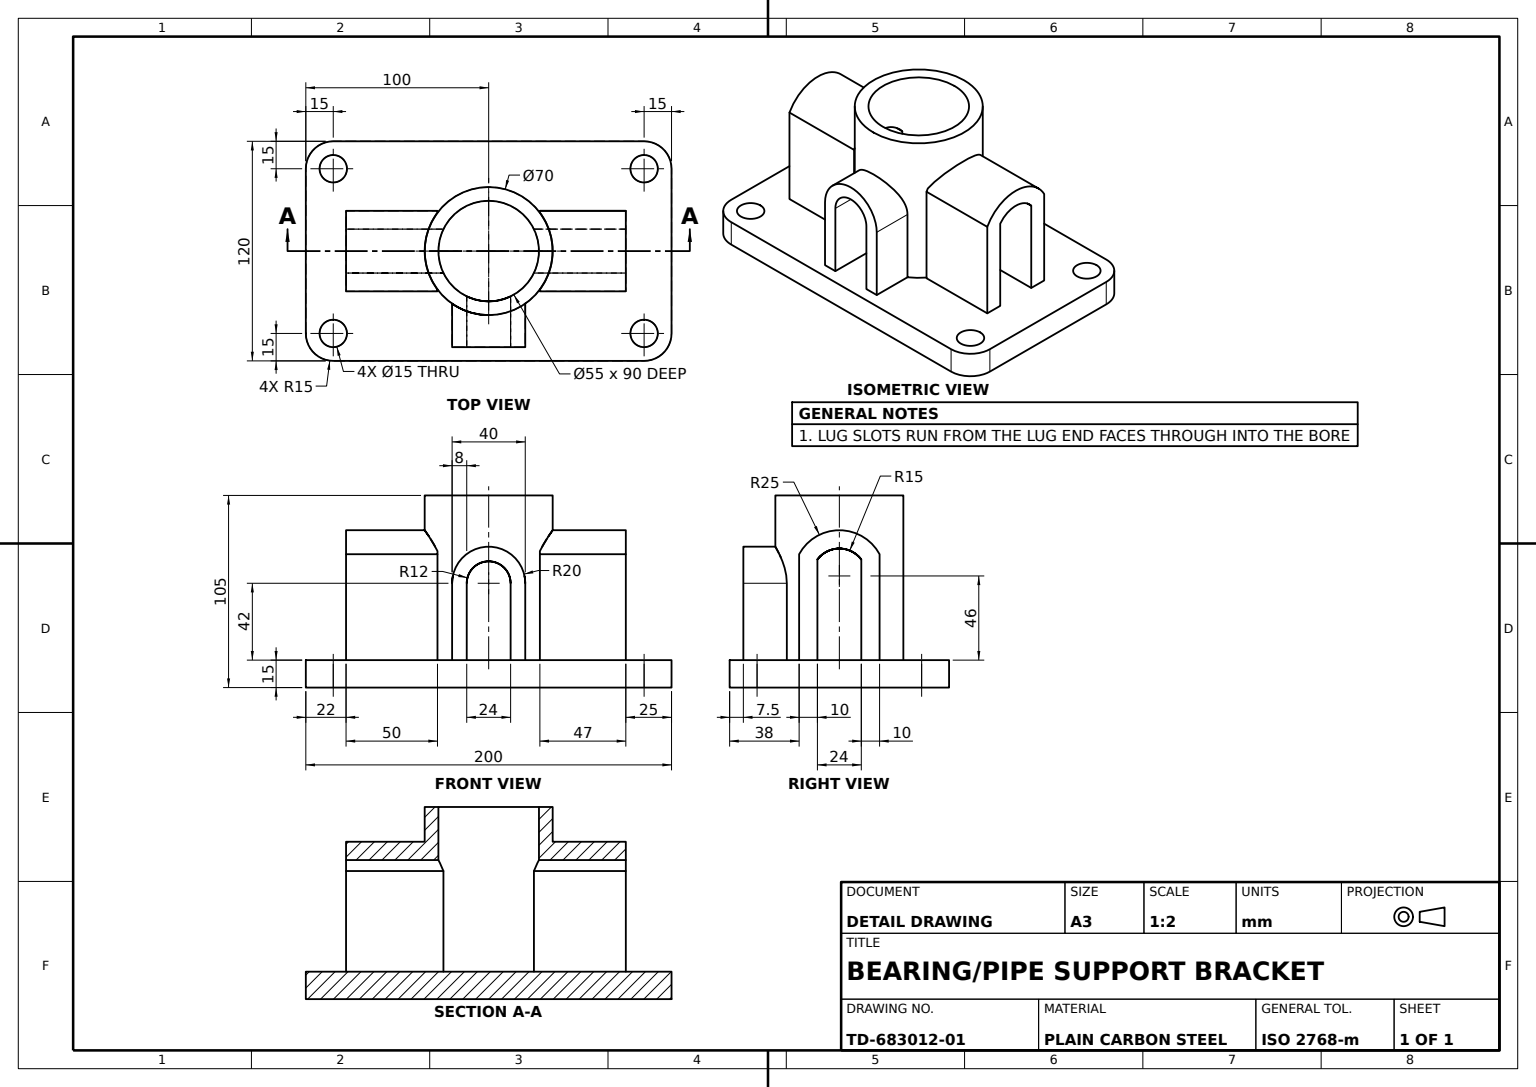
SolidWorks part; units mm, degrees
material "Plain Carbon Steel"
ref_plane "Front Plane" through (0, 0, 0) normal (0, 0, 1) x (1, 0, 0)
ref_plane "Top Plane" through (0, 0, 0) normal (0, 1, 0) x (1, 0, 0)
ref_plane "Right Plane" through (0, 0, 0) normal (1, 0, 0) x (0, 0, -1)
sketch "Base Plate Sketch" plane through (0, 0, 0) normal (0, 1, 0) x (1, 0, 0)
  line L1 (-85, -60) -> (85, -60)
  line L2 (-100, -45) -> (-100, 45)
  line L3 (-85, 60) -> (85, 60)
  line L4 (100, -45) -> (100, 45)
  line L5 (-100, -60) -> (100, 60) construction
  line L6 (-100, 60) -> (100, -60) construction
  arc A0 (-85, -60) -> (-100, -45) centre (-85, -45) cw
  arc A1 (100, -45) -> (85, -60) centre (85, -45) cw
  arc A2 (100, 45) -> (85, 60) centre (85, 45) ccw
  arc A3 (-85, 60) -> (-100, 45) centre (-85, 45) ccw
  circle A4 centre (-85, 45) radius 7.5
  circle A5 centre (85, 45) radius 7.5
  circle A6 centre (85, -45) radius 7.5
  circle A7 centre (-85, -45) radius 7.5
  point P0 (0, 0)
  dimension "D3" = 15
  dimension "D4" = 15
  dimension "D5" = 15
  dimension "D6" = 15
  dimension "D7" = 15
  dimension "D1" = 120
  dimension "D2" = 200
extrude "Base Plate 200x120x15" add sketch "Base Plate Sketch" along normal blind 15
sketch "Tube Boss Sketch" plane through (0, 15, 0) normal (0, 1, 0) x (1, 0, 0)
  circle A0 centre (0, 0) radius 35
  circle A1 centre (0, 0) radius 27.5
  dimension "D1" = 35
  dimension "D2" = 55
extrude "Tube Boss Ø55 Bore Ø35" add sketch "Tube Boss Sketch" along normal blind 90
ref_plane "Plane1" through (0, 0, 52.5) normal (0, 0, 1) x (1, 0, 0)
sketch "Front Lug Sketch" plane through (0, 0, 52.5) normal (0, 0, 1) x (1, 0, 0)
  line L0 (-12, 15) -> (-12, 57)
  line L1 (-85, 15) -> (85, 15) construction
  line L2 (-20, 15) -> (-20, 57)
  line L3 (12, 57) -> (12, 15)
  line L4 (20, 57) -> (20, 15)
  line L5 (-20, 15) -> (-12, 15)
  line L6 (12, 15) -> (20, 15)
  arc A0 (-12, 57) -> (12, 57) centre (0, 57) cw
  arc A1 (-20, 57) -> (20, 57) centre (0, 57) cw
  dimension "D2" = 12
  dimension "D4" = 42
  dimension "D1" = 24
  dimension "D3" = 8
extrude "Front Lug" add sketch "Front Lug Sketch" against normal blind 24 contours L4 L6 L3 A0 L0 L5 L2 A1
sketch "Front Lug Cut Sketch" plane through (0, 0, 52.5) normal (0, 0, 1) x (1, 0, 0)
  line L0 (12, 57) -> (12, 15) construction
  line L1 (-12, 57) -> (-12, 15) construction
  line L2 (12, 57) -> (12, 15)
  line L3 (-12, 57) -> (-12, 15)
  line L4 (-12, 15) -> (12, 15)
  arc A0 (12, 57) -> (-12, 57) centre (0, 57) ccw construction
  arc A1 (12, 57) -> (-12, 57) centre (0, 57) ccw construction
  arc A2 (12, 57) -> (-12, 57) centre (0, 57) ccw
  arc A3 (12, 57) -> (-12, 57) centre (0, 57) ccw
  line M4 (-12, 15) -> (-12, 57)
  arc M5 (-12, 57) -> (12, 57) centre (0, 57) cw
  line M6 (12, 57) -> (12, 15)
extrude "Front Lug Cut" cut sketch "Front Lug Cut Sketch" against normal blind 40 contours L4 M4 M6 M5
ref_plane "Plane2" through (-75, 0, 0) normal (-1, 0, 0) x (0, 0, 1)
sketch "Side Lug A Sketch" plane through (-75, 0, 0) normal (-1, 0, 0) x (0, 0, 1)
  line L0 (-12, 15) -> (-12, 70)
  line L1 (-45, 15) -> (45, 15) construction
  line L2 (-22, 15) -> (-22, 72.8743)
  line L3 (12, 70) -> (12, 15)
  line L4 (22, 72.8743) -> (22, 15)
  line L5 (-22, 15) -> (-12, 15)
  line L6 (12, 15) -> (22, 15)
  arc A0 (-12, 70) -> (12, 70) centre (0, 61) cw
  arc A1 (-22, 72.8743) -> (22, 72.8743) centre (0, 61) cw
  dimension "D2" = 15
  dimension "D1" = 24
  dimension "D3" = 55
  dimension "D4" = 55
  dimension "D5" = 10
extrude "Side Lug A" add sketch "Side Lug A Sketch" against normal blind 47 and the other way blind 3
sketch "Side Lug A Slot Sketch" plane through (-78, 0, 0) normal (-1, 0, 0) x (0, 0, 1)
  line L0 (12, 70) -> (12, 15) construction
  line L1 (-12, 15) -> (-12, 70) construction
  line L2 (12, 70) -> (12, 15)
  line L3 (-12, 15) -> (-12, 70)
  line L4 (-12, 15) -> (12, 15)
  arc A0 (12, 70) -> (-12, 70) centre (0, 61) ccw construction
  arc A1 (12, 70) -> (-12, 70) centre (0, 61) ccw
extrude "Side Lug A Slot" cut sketch "Side Lug A Slot Sketch" against normal blind 73
ref_plane "Plane3" through (75, 0, 0) normal (1, 0, 0) x (0, 0, -1)
sketch "Side Lug B Sketch" plane through (75, 0, 0) normal (1, 0, 0) x (0, 0, -1)
  line L0 (-12, 15) -> (-12, 70)
  line L1 (-45, 15) -> (45, 15) construction
  line L2 (-22, 15) -> (-22, 72.8743)
  line L3 (12, 70) -> (12, 15)
  line L4 (22, 72.8743) -> (22, 15)
  line L5 (-22, 15) -> (-12, 15)
  line L6 (12, 15) -> (22, 15)
  arc A0 (-12, 70) -> (12, 70) centre (0, 61) cw
  arc A1 (-22, 72.8743) -> (22, 72.8743) centre (0, 61) cw
  dimension "D2" = 15
  dimension "D5" = 55
  dimension "D1" = 24
  dimension "D3" = 55
  dimension "D4" = 10
extrude "Side Lug B" add sketch "Side Lug B Sketch" against normal blind 47
sketch "Side Lug B Slot Sketch" plane through (75, 0, 0) normal (1, 0, 0) x (0, 0, -1)
  line L0 (12, 15) -> (12, 70) construction
  line L1 (-12, 70) -> (-12, 15) construction
  line L2 (12, 15) -> (12, 70)
  line L3 (-12, 70) -> (-12, 15)
  line L4 (-12, 15) -> (12, 15)
  arc A0 (12, 70) -> (-12, 70) centre (0, 61) ccw construction
  arc A1 (12, 70) -> (-12, 70) centre (0, 61) ccw
extrude "Side Lug B Slot" cut sketch "Side Lug B Slot Sketch" against normal blind 67
